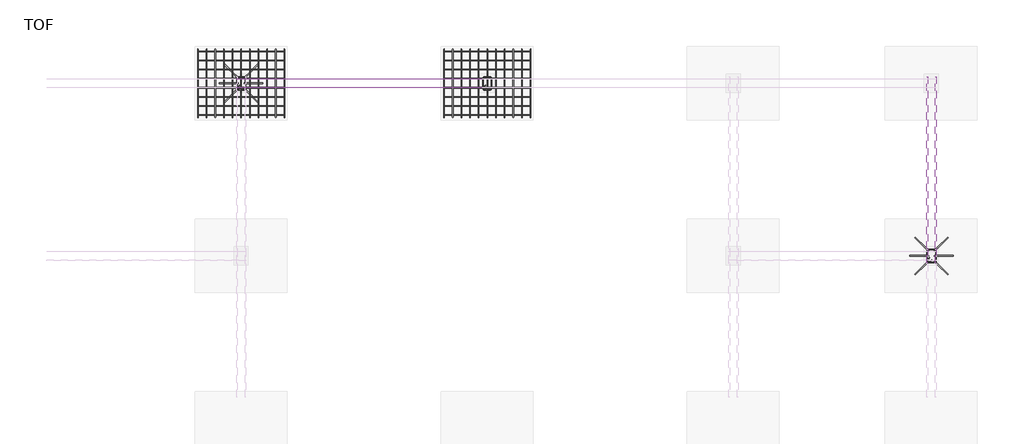
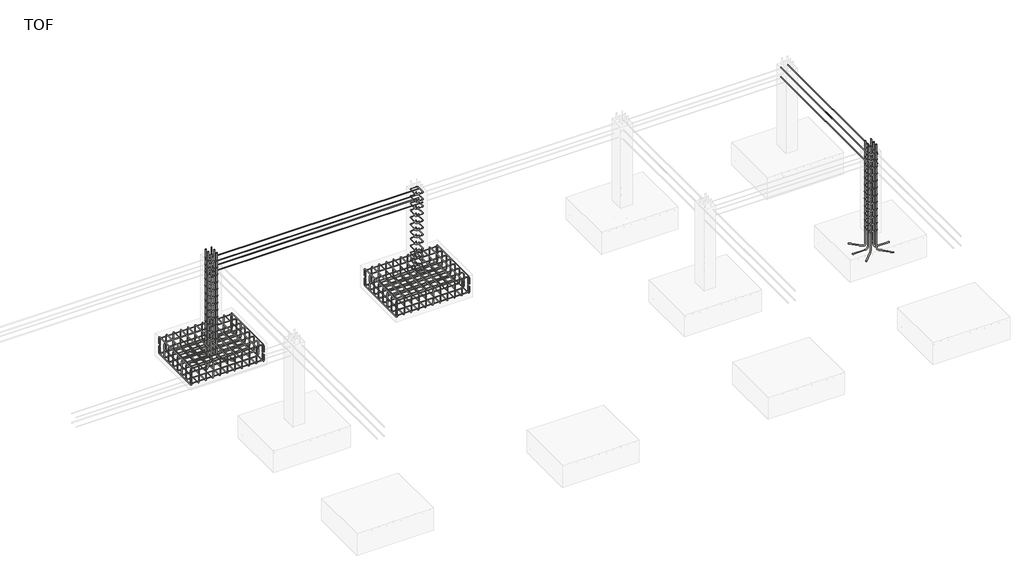
# One storey, part 9 of 10: 31 reinforcing bars.
"""IFC4 building model written with IfcOpenShell, lengths in millimetres."""

from ifc_helpers import new_model, si_unit, point, frame, origin, place, context, project, spatial, polyline, circle_curve, trimmed, segment, composite_curve, source, transform, mapped, element, save
from ifc_brep_helpers import swept_disk

model = new_model("IFC4")

# Units and contexts
model_context = context("Model", 3, world=origin())
ifc_project = project(units=[si_unit("LENGTHUNIT", "METRE", prefix="MILLI")], contexts=[model_context])

# Site, building, storey
site = spatial("IfcSite", under=ifc_project)
building = spatial("IfcBuilding", under=site)
storey = spatial("IfcBuildingStorey", under=building, Name="TOF", Elevation=-1828.8)

# Reinforcing bars
placement = place(None, origin())
reinforcing_bar_shape = source(origin(), model_context, "Body", "SolidModel", [
    swept_disk(composite_curve([segment(polyline([(2315.2782143, -7144.6267376, -2018.8), (2315.2782143, -7144.6267376, -1908.8)]), True, "CONTINUOUS"), segment(trimmed(circle_curve(frame((2315.2782143, -7179.6267376, -1908.8), z_axis=(1.0, 0.0, 0.0), x_axis=(0.0, 35.0, 0.0)), 35.0), [point((2315.2782143, -7144.6267376, -1908.8))], [point((2315.2782143, -7179.6267376, -1873.8))], True, "CARTESIAN"), True, "CONTINUOUS"), segment(polyline([(2315.2782143, -7179.6267376, -1873.8), (2315.2782143, -8219.6267376, -1873.8)]), True, "CONTINUOUS"), segment(trimmed(circle_curve(frame((2315.2782143, -8219.6267376, -1908.8), z_axis=(1.0, 0.0, 0.0), x_axis=(0.0, 0.0, 35.0)), 35.0), [point((2315.2782143, -8219.6267376, -1873.8))], [point((2315.2782143, -8254.6267376, -1908.8))], True, "CARTESIAN"), True, "CONTINUOUS"), segment(polyline([(2315.2782143, -8254.6267376, -1908.8), (2315.2782143, -8254.6267376, -2018.8)]), True, "CONTINUOUS")], self_intersect=False), 5.0),
])
element("IfcReinforcingBar", 1, at=placement, inside=storey, context=model_context, shape_type="MappedRepresentation", body=[
    mapped(reinforcing_bar_shape, transform((0.0, 0.0, 0.0), x_axis=(1.0, 0.0, 0.0), y_axis=(0.0, 1.0, 0.0), z_axis=(0.0, 0.0, 1.0))),
    mapped(reinforcing_bar_shape, transform((-141.0, 0.0, 0.0), x_axis=(1.0, 0.0, 0.0), y_axis=(0.0, 1.0, 0.0), z_axis=(0.0, 0.0, 1.0))),
    mapped(reinforcing_bar_shape, transform((-282.0, 0.0, 0.0), x_axis=(1.0, 0.0, 0.0), y_axis=(0.0, 1.0, 0.0), z_axis=(0.0, 0.0, 1.0))),
    mapped(reinforcing_bar_shape, transform((-423.0, 0.0, 0.0), x_axis=(1.0, 0.0, 0.0), y_axis=(0.0, 1.0, 0.0), z_axis=(0.0, 0.0, 1.0))),
    mapped(reinforcing_bar_shape, transform((-564.0, 0.0, 0.0), x_axis=(1.0, 0.0, 0.0), y_axis=(0.0, 1.0, 0.0), z_axis=(0.0, 0.0, 1.0))),
    mapped(reinforcing_bar_shape, transform((-705.0, 0.0, 0.0), x_axis=(1.0, 0.0, 0.0), y_axis=(0.0, 1.0, 0.0), z_axis=(0.0, 0.0, 1.0))),
    mapped(reinforcing_bar_shape, transform((-846.0, 0.0, 0.0), x_axis=(1.0, 0.0, 0.0), y_axis=(0.0, 1.0, 0.0), z_axis=(0.0, 0.0, 1.0))),
    mapped(reinforcing_bar_shape, transform((-987.0, 0.0, 0.0), x_axis=(1.0, 0.0, 0.0), y_axis=(0.0, 1.0, 0.0), z_axis=(0.0, 0.0, 1.0))),
    mapped(reinforcing_bar_shape, transform((-1128.0, 0.0, 0.0), x_axis=(1.0, 0.0, 0.0), y_axis=(0.0, 1.0, 0.0), z_axis=(0.0, 0.0, 1.0))),
    mapped(reinforcing_bar_shape, transform((-1269.0, 0.0, 0.0), x_axis=(1.0, 0.0, 0.0), y_axis=(0.0, 1.0, 0.0), z_axis=(0.0, 0.0, 1.0))),
    mapped(reinforcing_bar_shape, transform((-1410.0, 0.0, 0.0), x_axis=(1.0, 0.0, 0.0), y_axis=(0.0, 1.0, 0.0), z_axis=(0.0, 0.0, 1.0))),
])
reinforcing_bar_2_shape = source(origin(), model_context, "Body", "SolidModel", [
    swept_disk(composite_curve([segment(polyline([(2315.2782143, -8254.6267376, -2077.5233378), (2315.2782143, -8254.6267376, -2187.5233378)]), True, "CONTINUOUS"), segment(trimmed(circle_curve(frame((2315.2782143, -8219.6267376, -2187.5233378), z_axis=(1.0, 0.0, 0.0), x_axis=(0.0, -35.0, 0.0)), 35.0), [point((2315.2782143, -8254.6267376, -2187.5233378))], [point((2315.2782143, -8219.6267376, -2222.5233378))], True, "CARTESIAN"), True, "CONTINUOUS"), segment(polyline([(2315.2782143, -8219.6267376, -2222.5233378), (2315.2782143, -7179.6267376, -2222.5233378)]), True, "CONTINUOUS"), segment(trimmed(circle_curve(frame((2315.2782143, -7179.6267376, -2187.5233378), z_axis=(1.0, 0.0, 0.0), x_axis=(0.0, 0.0, -35.0)), 35.0), [point((2315.2782143, -7179.6267376, -2222.5233378))], [point((2315.2782143, -7144.6267376, -2187.5233378))], True, "CARTESIAN"), True, "CONTINUOUS"), segment(polyline([(2315.2782143, -7144.6267376, -2187.5233378), (2315.2782143, -7144.6267376, -2077.5233378)]), True, "CONTINUOUS")], self_intersect=False), 5.0),
])
element("IfcReinforcingBar", 2, at=placement, inside=storey, context=model_context, shape_type="MappedRepresentation", body=[
    mapped(reinforcing_bar_2_shape, transform((0.0, 0.0, 0.0), x_axis=(1.0, 0.0, 0.0), y_axis=(0.0, 1.0, 0.0), z_axis=(0.0, 0.0, 1.0))),
    mapped(reinforcing_bar_2_shape, transform((-141.0, 0.0, 0.0), x_axis=(1.0, 0.0, 0.0), y_axis=(0.0, 1.0, 0.0), z_axis=(0.0, 0.0, 1.0))),
    mapped(reinforcing_bar_2_shape, transform((-282.0, 0.0, 0.0), x_axis=(1.0, 0.0, 0.0), y_axis=(0.0, 1.0, 0.0), z_axis=(0.0, 0.0, 1.0))),
    mapped(reinforcing_bar_2_shape, transform((-423.0, 0.0, 0.0), x_axis=(1.0, 0.0, 0.0), y_axis=(0.0, 1.0, 0.0), z_axis=(0.0, 0.0, 1.0))),
    mapped(reinforcing_bar_2_shape, transform((-564.0, 0.0, 0.0), x_axis=(1.0, 0.0, 0.0), y_axis=(0.0, 1.0, 0.0), z_axis=(0.0, 0.0, 1.0))),
    mapped(reinforcing_bar_2_shape, transform((-705.0, 0.0, 0.0), x_axis=(1.0, 0.0, 0.0), y_axis=(0.0, 1.0, 0.0), z_axis=(0.0, 0.0, 1.0))),
    mapped(reinforcing_bar_2_shape, transform((-846.0, 0.0, 0.0), x_axis=(1.0, 0.0, 0.0), y_axis=(0.0, 1.0, 0.0), z_axis=(0.0, 0.0, 1.0))),
    mapped(reinforcing_bar_2_shape, transform((-987.0, 0.0, 0.0), x_axis=(1.0, 0.0, 0.0), y_axis=(0.0, 1.0, 0.0), z_axis=(0.0, 0.0, 1.0))),
    mapped(reinforcing_bar_2_shape, transform((-1128.0, 0.0, 0.0), x_axis=(1.0, 0.0, 0.0), y_axis=(0.0, 1.0, 0.0), z_axis=(0.0, 0.0, 1.0))),
    mapped(reinforcing_bar_2_shape, transform((-1269.0, 0.0, 0.0), x_axis=(1.0, 0.0, 0.0), y_axis=(0.0, 1.0, 0.0), z_axis=(0.0, 0.0, 1.0))),
    mapped(reinforcing_bar_2_shape, transform((-1410.0, 0.0, 0.0), x_axis=(1.0, 0.0, 0.0), y_axis=(0.0, 1.0, 0.0), z_axis=(0.0, 0.0, 1.0))),
])
reinforcing_bar_3_shape = source(origin(), model_context, "Body", "SolidModel", [
    swept_disk(composite_curve([segment(polyline([(2315.2782143, -7179.6861459, -2066.1776706), (2315.2782143, -7179.6861459, -2176.1776706)]), True, "CONTINUOUS"), segment(trimmed(circle_curve(frame((2280.2782143, -7179.6861459, -2176.1776706), z_axis=(0.0, 1.0, 0.0), x_axis=(35.0, 0.0, 0.0)), 35.0), [point((2315.2782143, -7179.6861459, -2176.1776706))], [point((2280.2782143, -7179.6861459, -2211.1776706))], True, "CARTESIAN"), True, "CONTINUOUS"), segment(polyline([(2280.2782143, -7179.6861459, -2211.1776706), (940.2782143, -7179.6861459, -2211.1776706)]), True, "CONTINUOUS"), segment(trimmed(circle_curve(frame((940.2782143, -7179.6861459, -2176.1776706), z_axis=(0.0, 1.0, 0.0), x_axis=(0.0, 0.0, -35.0)), 35.0), [point((940.2782143, -7179.6861459, -2211.1776706))], [point((905.2782143, -7179.6861459, -2176.1776706))], True, "CARTESIAN"), True, "CONTINUOUS"), segment(polyline([(905.2782143, -7179.6861459, -2176.1776706), (905.2782143, -7179.6861459, -2066.1776706)]), True, "CONTINUOUS")], self_intersect=False), 5.0),
])
element("IfcReinforcingBar", 3, at=placement, inside=storey, context=model_context, shape_type="MappedRepresentation", body=[
    mapped(reinforcing_bar_3_shape, transform((0.0, 0.0, 0.0), x_axis=(1.0, 0.0, 0.0), y_axis=(0.0, 1.0, 0.0), z_axis=(0.0, 0.0, 1.0))),
    mapped(reinforcing_bar_3_shape, transform((0.0, -148.0321606, 0.0), x_axis=(1.0, 0.0, 0.0), y_axis=(0.0, 1.0, 0.0), z_axis=(0.0, 0.0, 1.0))),
    mapped(reinforcing_bar_3_shape, transform((0.0, -296.0643211, 0.0), x_axis=(1.0, 0.0, 0.0), y_axis=(0.0, 1.0, 0.0), z_axis=(0.0, 0.0, 1.0))),
    mapped(reinforcing_bar_3_shape, transform((0.0, -444.0964817, 0.0), x_axis=(1.0, 0.0, 0.0), y_axis=(0.0, 1.0, 0.0), z_axis=(0.0, 0.0, 1.0))),
    mapped(reinforcing_bar_3_shape, transform((0.0, -592.1286423, 0.0), x_axis=(1.0, 0.0, 0.0), y_axis=(0.0, 1.0, 0.0), z_axis=(0.0, 0.0, 1.0))),
    mapped(reinforcing_bar_3_shape, transform((0.0, -740.1608029, 0.0), x_axis=(1.0, 0.0, 0.0), y_axis=(0.0, 1.0, 0.0), z_axis=(0.0, 0.0, 1.0))),
    mapped(reinforcing_bar_3_shape, transform((0.0, -888.1929634, 0.0), x_axis=(1.0, 0.0, 0.0), y_axis=(0.0, 1.0, 0.0), z_axis=(0.0, 0.0, 1.0))),
    mapped(reinforcing_bar_3_shape, transform((0.0, -1036.225124, 0.0), x_axis=(1.0, 0.0, 0.0), y_axis=(0.0, 1.0, 0.0), z_axis=(0.0, 0.0, 1.0))),
])
reinforcing_bar_4_shape = source(origin(), model_context, "Body", "SolidModel", [
    swept_disk(composite_curve([segment(polyline([(2315.2782143, -8215.9112699, -2039.256778), (2315.2782143, -8215.9112699, -1929.256778)]), True, "CONTINUOUS"), segment(trimmed(circle_curve(frame((2280.2782143, -8215.9112699, -1929.256778), z_axis=(0.0, -1.0, 0.0), x_axis=(35.0, 0.0, 0.0)), 35.0), [point((2315.2782143, -8215.9112699, -1929.256778))], [point((2280.2782143, -8215.9112699, -1894.256778))], True, "CARTESIAN"), True, "CONTINUOUS"), segment(polyline([(2280.2782143, -8215.9112699, -1894.256778), (940.2782143, -8215.9112699, -1894.256778)]), True, "CONTINUOUS"), segment(trimmed(circle_curve(frame((940.2782143, -8215.9112699, -1929.256778), z_axis=(0.0, -1.0, 0.0), x_axis=(0.0, 0.0, 35.0)), 35.0), [point((940.2782143, -8215.9112699, -1894.256778))], [point((905.2782143, -8215.9112699, -1929.256778))], True, "CARTESIAN"), True, "CONTINUOUS"), segment(polyline([(905.2782143, -8215.9112699, -1929.256778), (905.2782143, -8215.9112699, -2039.256778)]), True, "CONTINUOUS")], self_intersect=False), 5.0),
])
element("IfcReinforcingBar", 4, at=placement, inside=storey, context=model_context, shape_type="MappedRepresentation", body=[
    mapped(reinforcing_bar_4_shape, transform((0.0, 0.0, 0.0), x_axis=(1.0, 0.0, 0.0), y_axis=(0.0, 1.0, 0.0), z_axis=(0.0, 0.0, 1.0))),
    mapped(reinforcing_bar_4_shape, transform((0.0, 148.0321606, 0.0), x_axis=(1.0, 0.0, 0.0), y_axis=(0.0, 1.0, 0.0), z_axis=(0.0, 0.0, 1.0))),
    mapped(reinforcing_bar_4_shape, transform((0.0, 296.0643211, 0.0), x_axis=(1.0, 0.0, 0.0), y_axis=(0.0, 1.0, 0.0), z_axis=(0.0, 0.0, 1.0))),
    mapped(reinforcing_bar_4_shape, transform((0.0, 444.0964817, 0.0), x_axis=(1.0, 0.0, 0.0), y_axis=(0.0, 1.0, 0.0), z_axis=(0.0, 0.0, 1.0))),
    mapped(reinforcing_bar_4_shape, transform((0.0, 592.1286423, 0.0), x_axis=(1.0, 0.0, 0.0), y_axis=(0.0, 1.0, 0.0), z_axis=(0.0, 0.0, 1.0))),
    mapped(reinforcing_bar_4_shape, transform((0.0, 740.1608029, 0.0), x_axis=(1.0, 0.0, 0.0), y_axis=(0.0, 1.0, 0.0), z_axis=(0.0, 0.0, 1.0))),
    mapped(reinforcing_bar_4_shape, transform((0.0, 888.1929634, 0.0), x_axis=(1.0, 0.0, 0.0), y_axis=(0.0, 1.0, 0.0), z_axis=(0.0, 0.0, 1.0))),
    mapped(reinforcing_bar_4_shape, transform((0.0, 1036.225124, 0.0), x_axis=(1.0, 0.0, 0.0), y_axis=(0.0, 1.0, 0.0), z_axis=(0.0, 0.0, 1.0))),
])
reinforcing_bar_5_shape = source(origin(), model_context, "Body", "SolidModel", [
    swept_disk(composite_curve([segment(polyline([(6330.2782143, -7144.6267376, -2018.8), (6330.2782143, -7144.6267376, -1908.8)]), True, "CONTINUOUS"), segment(trimmed(circle_curve(frame((6330.2782143, -7179.6267376, -1908.8), z_axis=(1.0, 0.0, 0.0), x_axis=(0.0, 35.0, 0.0)), 35.0), [point((6330.2782143, -7144.6267376, -1908.8))], [point((6330.2782143, -7179.6267376, -1873.8))], True, "CARTESIAN"), True, "CONTINUOUS"), segment(polyline([(6330.2782143, -7179.6267376, -1873.8), (6330.2782143, -8219.6267376, -1873.8)]), True, "CONTINUOUS"), segment(trimmed(circle_curve(frame((6330.2782143, -8219.6267376, -1908.8), z_axis=(1.0, 0.0, 0.0), x_axis=(0.0, 0.0, 35.0)), 35.0), [point((6330.2782143, -8219.6267376, -1873.8))], [point((6330.2782143, -8254.6267376, -1908.8))], True, "CARTESIAN"), True, "CONTINUOUS"), segment(polyline([(6330.2782143, -8254.6267376, -1908.8), (6330.2782143, -8254.6267376, -2018.8)]), True, "CONTINUOUS")], self_intersect=False), 5.0),
])
element("IfcReinforcingBar", 5, at=placement, inside=storey, context=model_context, shape_type="MappedRepresentation", body=[
    mapped(reinforcing_bar_5_shape, transform((0.0, 0.0, 0.0), x_axis=(1.0, 0.0, 0.0), y_axis=(0.0, 1.0, 0.0), z_axis=(0.0, 0.0, 1.0))),
    mapped(reinforcing_bar_5_shape, transform((-141.0, 0.0, 0.0), x_axis=(1.0, 0.0, 0.0), y_axis=(0.0, 1.0, 0.0), z_axis=(0.0, 0.0, 1.0))),
    mapped(reinforcing_bar_5_shape, transform((-282.0, 0.0, 0.0), x_axis=(1.0, 0.0, 0.0), y_axis=(0.0, 1.0, 0.0), z_axis=(0.0, 0.0, 1.0))),
    mapped(reinforcing_bar_5_shape, transform((-423.0, 0.0, 0.0), x_axis=(1.0, 0.0, 0.0), y_axis=(0.0, 1.0, 0.0), z_axis=(0.0, 0.0, 1.0))),
    mapped(reinforcing_bar_5_shape, transform((-564.0, 0.0, 0.0), x_axis=(1.0, 0.0, 0.0), y_axis=(0.0, 1.0, 0.0), z_axis=(0.0, 0.0, 1.0))),
    mapped(reinforcing_bar_5_shape, transform((-705.0, 0.0, 0.0), x_axis=(1.0, 0.0, 0.0), y_axis=(0.0, 1.0, 0.0), z_axis=(0.0, 0.0, 1.0))),
    mapped(reinforcing_bar_5_shape, transform((-846.0, 0.0, 0.0), x_axis=(1.0, 0.0, 0.0), y_axis=(0.0, 1.0, 0.0), z_axis=(0.0, 0.0, 1.0))),
    mapped(reinforcing_bar_5_shape, transform((-987.0, 0.0, 0.0), x_axis=(1.0, 0.0, 0.0), y_axis=(0.0, 1.0, 0.0), z_axis=(0.0, 0.0, 1.0))),
    mapped(reinforcing_bar_5_shape, transform((-1128.0, 0.0, 0.0), x_axis=(1.0, 0.0, 0.0), y_axis=(0.0, 1.0, 0.0), z_axis=(0.0, 0.0, 1.0))),
    mapped(reinforcing_bar_5_shape, transform((-1269.0, 0.0, 0.0), x_axis=(1.0, 0.0, 0.0), y_axis=(0.0, 1.0, 0.0), z_axis=(0.0, 0.0, 1.0))),
    mapped(reinforcing_bar_5_shape, transform((-1410.0, 0.0, 0.0), x_axis=(1.0, 0.0, 0.0), y_axis=(0.0, 1.0, 0.0), z_axis=(0.0, 0.0, 1.0))),
])
reinforcing_bar_6_shape = source(origin(), model_context, "Body", "SolidModel", [
    swept_disk(composite_curve([segment(polyline([(6330.2782143, -8254.6267376, -2077.5233378), (6330.2782143, -8254.6267376, -2187.5233378)]), True, "CONTINUOUS"), segment(trimmed(circle_curve(frame((6330.2782143, -8219.6267376, -2187.5233378), z_axis=(1.0, 0.0, 0.0), x_axis=(0.0, -35.0, 0.0)), 35.0), [point((6330.2782143, -8254.6267376, -2187.5233378))], [point((6330.2782143, -8219.6267376, -2222.5233378))], True, "CARTESIAN"), True, "CONTINUOUS"), segment(polyline([(6330.2782143, -8219.6267376, -2222.5233378), (6330.2782143, -7179.6267376, -2222.5233378)]), True, "CONTINUOUS"), segment(trimmed(circle_curve(frame((6330.2782143, -7179.6267376, -2187.5233378), z_axis=(1.0, 0.0, 0.0), x_axis=(0.0, 0.0, -35.0)), 35.0), [point((6330.2782143, -7179.6267376, -2222.5233378))], [point((6330.2782143, -7144.6267376, -2187.5233378))], True, "CARTESIAN"), True, "CONTINUOUS"), segment(polyline([(6330.2782143, -7144.6267376, -2187.5233378), (6330.2782143, -7144.6267376, -2077.5233378)]), True, "CONTINUOUS")], self_intersect=False), 5.0),
])
element("IfcReinforcingBar", 6, at=placement, inside=storey, context=model_context, shape_type="MappedRepresentation", body=[
    mapped(reinforcing_bar_6_shape, transform((0.0, 0.0, 0.0), x_axis=(1.0, 0.0, 0.0), y_axis=(0.0, 1.0, 0.0), z_axis=(0.0, 0.0, 1.0))),
    mapped(reinforcing_bar_6_shape, transform((-141.0, 0.0, 0.0), x_axis=(1.0, 0.0, 0.0), y_axis=(0.0, 1.0, 0.0), z_axis=(0.0, 0.0, 1.0))),
    mapped(reinforcing_bar_6_shape, transform((-282.0, 0.0, 0.0), x_axis=(1.0, 0.0, 0.0), y_axis=(0.0, 1.0, 0.0), z_axis=(0.0, 0.0, 1.0))),
    mapped(reinforcing_bar_6_shape, transform((-423.0, 0.0, 0.0), x_axis=(1.0, 0.0, 0.0), y_axis=(0.0, 1.0, 0.0), z_axis=(0.0, 0.0, 1.0))),
    mapped(reinforcing_bar_6_shape, transform((-564.0, 0.0, 0.0), x_axis=(1.0, 0.0, 0.0), y_axis=(0.0, 1.0, 0.0), z_axis=(0.0, 0.0, 1.0))),
    mapped(reinforcing_bar_6_shape, transform((-705.0, 0.0, 0.0), x_axis=(1.0, 0.0, 0.0), y_axis=(0.0, 1.0, 0.0), z_axis=(0.0, 0.0, 1.0))),
    mapped(reinforcing_bar_6_shape, transform((-846.0, 0.0, 0.0), x_axis=(1.0, 0.0, 0.0), y_axis=(0.0, 1.0, 0.0), z_axis=(0.0, 0.0, 1.0))),
    mapped(reinforcing_bar_6_shape, transform((-987.0, 0.0, 0.0), x_axis=(1.0, 0.0, 0.0), y_axis=(0.0, 1.0, 0.0), z_axis=(0.0, 0.0, 1.0))),
    mapped(reinforcing_bar_6_shape, transform((-1128.0, 0.0, 0.0), x_axis=(1.0, 0.0, 0.0), y_axis=(0.0, 1.0, 0.0), z_axis=(0.0, 0.0, 1.0))),
    mapped(reinforcing_bar_6_shape, transform((-1269.0, 0.0, 0.0), x_axis=(1.0, 0.0, 0.0), y_axis=(0.0, 1.0, 0.0), z_axis=(0.0, 0.0, 1.0))),
    mapped(reinforcing_bar_6_shape, transform((-1410.0, 0.0, 0.0), x_axis=(1.0, 0.0, 0.0), y_axis=(0.0, 1.0, 0.0), z_axis=(0.0, 0.0, 1.0))),
])
reinforcing_bar_7_shape = source(origin(), model_context, "Body", "SolidModel", [
    swept_disk(composite_curve([segment(polyline([(6330.2782143, -7179.6861459, -2066.1776706), (6330.2782143, -7179.6861459, -2176.1776706)]), True, "CONTINUOUS"), segment(trimmed(circle_curve(frame((6295.2782143, -7179.6861459, -2176.1776706), z_axis=(0.0, 1.0, 0.0), x_axis=(35.0, 0.0, 0.0)), 35.0), [point((6330.2782143, -7179.6861459, -2176.1776706))], [point((6295.2782143, -7179.6861459, -2211.1776706))], True, "CARTESIAN"), True, "CONTINUOUS"), segment(polyline([(6295.2782143, -7179.6861459, -2211.1776706), (4955.2782143, -7179.6861459, -2211.1776706)]), True, "CONTINUOUS"), segment(trimmed(circle_curve(frame((4955.2782143, -7179.6861459, -2176.1776706), z_axis=(0.0, 1.0, 0.0), x_axis=(0.0, 0.0, -35.0)), 35.0), [point((4955.2782143, -7179.6861459, -2211.1776706))], [point((4920.2782143, -7179.6861459, -2176.1776706))], True, "CARTESIAN"), True, "CONTINUOUS"), segment(polyline([(4920.2782143, -7179.6861459, -2176.1776706), (4920.2782143, -7179.6861459, -2066.1776706)]), True, "CONTINUOUS")], self_intersect=False), 5.0),
])
element("IfcReinforcingBar", 7, at=placement, inside=storey, context=model_context, shape_type="MappedRepresentation", body=[
    mapped(reinforcing_bar_7_shape, transform((0.0, 0.0, 0.0), x_axis=(1.0, 0.0, 0.0), y_axis=(0.0, 1.0, 0.0), z_axis=(0.0, 0.0, 1.0))),
    mapped(reinforcing_bar_7_shape, transform((0.0, -148.0321606, 0.0), x_axis=(1.0, 0.0, 0.0), y_axis=(0.0, 1.0, 0.0), z_axis=(0.0, 0.0, 1.0))),
    mapped(reinforcing_bar_7_shape, transform((0.0, -296.0643211, 0.0), x_axis=(1.0, 0.0, 0.0), y_axis=(0.0, 1.0, 0.0), z_axis=(0.0, 0.0, 1.0))),
    mapped(reinforcing_bar_7_shape, transform((0.0, -444.0964817, 0.0), x_axis=(1.0, 0.0, 0.0), y_axis=(0.0, 1.0, 0.0), z_axis=(0.0, 0.0, 1.0))),
    mapped(reinforcing_bar_7_shape, transform((0.0, -592.1286423, 0.0), x_axis=(1.0, 0.0, 0.0), y_axis=(0.0, 1.0, 0.0), z_axis=(0.0, 0.0, 1.0))),
    mapped(reinforcing_bar_7_shape, transform((0.0, -740.1608029, 0.0), x_axis=(1.0, 0.0, 0.0), y_axis=(0.0, 1.0, 0.0), z_axis=(0.0, 0.0, 1.0))),
    mapped(reinforcing_bar_7_shape, transform((0.0, -888.1929634, 0.0), x_axis=(1.0, 0.0, 0.0), y_axis=(0.0, 1.0, 0.0), z_axis=(0.0, 0.0, 1.0))),
    mapped(reinforcing_bar_7_shape, transform((0.0, -1036.225124, 0.0), x_axis=(1.0, 0.0, 0.0), y_axis=(0.0, 1.0, 0.0), z_axis=(0.0, 0.0, 1.0))),
])
reinforcing_bar_8_shape = source(origin(), model_context, "Body", "SolidModel", [
    swept_disk(composite_curve([segment(polyline([(6330.2782143, -8215.9112699, -2039.256778), (6330.2782143, -8215.9112699, -1929.256778)]), True, "CONTINUOUS"), segment(trimmed(circle_curve(frame((6295.2782143, -8215.9112699, -1929.256778), z_axis=(0.0, -1.0, 0.0), x_axis=(35.0, 0.0, 0.0)), 35.0), [point((6330.2782143, -8215.9112699, -1929.256778))], [point((6295.2782143, -8215.9112699, -1894.256778))], True, "CARTESIAN"), True, "CONTINUOUS"), segment(polyline([(6295.2782143, -8215.9112699, -1894.256778), (4955.2782143, -8215.9112699, -1894.256778)]), True, "CONTINUOUS"), segment(trimmed(circle_curve(frame((4955.2782143, -8215.9112699, -1929.256778), z_axis=(0.0, -1.0, 0.0), x_axis=(0.0, 0.0, 35.0)), 35.0), [point((4955.2782143, -8215.9112699, -1894.256778))], [point((4920.2782143, -8215.9112699, -1929.256778))], True, "CARTESIAN"), True, "CONTINUOUS"), segment(polyline([(4920.2782143, -8215.9112699, -1929.256778), (4920.2782143, -8215.9112699, -2039.256778)]), True, "CONTINUOUS")], self_intersect=False), 5.0),
])
element("IfcReinforcingBar", 8, at=placement, inside=storey, context=model_context, shape_type="MappedRepresentation", body=[
    mapped(reinforcing_bar_8_shape, transform((0.0, 0.0, 0.0), x_axis=(1.0, 0.0, 0.0), y_axis=(0.0, 1.0, 0.0), z_axis=(0.0, 0.0, 1.0))),
    mapped(reinforcing_bar_8_shape, transform((0.0, 148.0321606, 0.0), x_axis=(1.0, 0.0, 0.0), y_axis=(0.0, 1.0, 0.0), z_axis=(0.0, 0.0, 1.0))),
    mapped(reinforcing_bar_8_shape, transform((0.0, 296.0643211, 0.0), x_axis=(1.0, 0.0, 0.0), y_axis=(0.0, 1.0, 0.0), z_axis=(0.0, 0.0, 1.0))),
    mapped(reinforcing_bar_8_shape, transform((0.0, 444.0964817, 0.0), x_axis=(1.0, 0.0, 0.0), y_axis=(0.0, 1.0, 0.0), z_axis=(0.0, 0.0, 1.0))),
    mapped(reinforcing_bar_8_shape, transform((0.0, 592.1286423, 0.0), x_axis=(1.0, 0.0, 0.0), y_axis=(0.0, 1.0, 0.0), z_axis=(0.0, 0.0, 1.0))),
    mapped(reinforcing_bar_8_shape, transform((0.0, 740.1608029, 0.0), x_axis=(1.0, 0.0, 0.0), y_axis=(0.0, 1.0, 0.0), z_axis=(0.0, 0.0, 1.0))),
    mapped(reinforcing_bar_8_shape, transform((0.0, 888.1929634, 0.0), x_axis=(1.0, 0.0, 0.0), y_axis=(0.0, 1.0, 0.0), z_axis=(0.0, 0.0, 1.0))),
    mapped(reinforcing_bar_8_shape, transform((0.0, 1036.225124, 0.0), x_axis=(1.0, 0.0, 0.0), y_axis=(0.0, 1.0, 0.0), z_axis=(0.0, 0.0, 1.0))),
])
reinforcing_bar_9_shape = source(origin(), model_context, "Body", "SolidModel", [
    swept_disk(composite_curve([segment(polyline([(12840.248777, -10545.7150493, -1784.8), (12806.3076515, -10579.6561748, -1784.8)]), True, "CONTINUOUS"), segment(trimmed(circle_curve(frame((12823.2782143, -10596.6267376, -1784.8), z_axis=(0.0, 0.0, 1.0), x_axis=(-16.970562800001062, 16.970562799999243, 0.0)), 24.0), [point((12806.3076515, -10579.6561748, -1784.8))], [point((12823.2782143, -10620.6267376, -1784.8))], True, "CARTESIAN"), True, "CONTINUOUS"), segment(polyline([(12823.2782143, -10620.6267376, -1784.8), (12917.2782143, -10620.6267376, -1784.8)]), True, "CONTINUOUS"), segment(trimmed(circle_curve(frame((12917.2782143, -10596.6267376, -1784.8), z_axis=(0.0, 0.0, 1.0), x_axis=(0.0, -24.0, 0.0)), 24.0), [point((12917.2782143, -10620.6267376, -1784.8))], [point((12941.2782143, -10596.6267376, -1784.8))], True, "CARTESIAN"), True, "CONTINUOUS"), segment(polyline([(12941.2782143, -10596.6267376, -1784.8), (12941.2782143, -10432.6267376, -1784.8)]), True, "CONTINUOUS"), segment(trimmed(circle_curve(frame((12917.3162115, -10432.6267376, -1786.149972), z_axis=(-0.05624883273897078, 0.0, 0.9984167811167355), x_axis=(23.962002800000846, 0.0, 1.3499719999999797)), 24.0), [point((12941.2782143, -10432.6267376, -1784.8))], [point((12917.3162115, -10408.6267376, -1786.149972))], True, "CARTESIAN"), True, "CONTINUOUS"), segment(polyline([(12917.3162115, -10408.6267376, -1786.149972), (12823.240217, -10408.6267376, -1791.450028)]), True, "CONTINUOUS"), segment(trimmed(circle_curve(frame((12823.240217, -10432.6267376, -1791.450028), z_axis=(-0.05624883273897078, 0.0, 0.9984167811167355), x_axis=(0.0, 24.0, 0.0)), 24.0), [point((12823.240217, -10408.6267376, -1791.450028))], [point((12799.2782143, -10432.6267376, -1792.8))], True, "CARTESIAN"), True, "CONTINUOUS"), segment(polyline([(12799.2782143, -10432.6267376, -1792.8), (12799.2782143, -10596.6267376, -1792.8)]), True, "CONTINUOUS"), segment(trimmed(circle_curve(frame((12823.2782143, -10596.6267376, -1792.8), z_axis=(0.0, 0.0, 1.0), x_axis=(-24.0, 0.0, 0.0)), 24.0), [point((12799.2782143, -10596.6267376, -1792.8))], [point((12840.248777, -10613.5973003, -1792.8))], True, "CARTESIAN"), True, "CONTINUOUS"), segment(polyline([(12840.248777, -10613.5973003, -1792.8), (12874.1899025, -10579.6561748, -1792.8)]), True, "CONTINUOUS")], self_intersect=False), 4.0),
])
element("IfcReinforcingBar", 9, at=placement, inside=storey, context=model_context, shape_type="MappedRepresentation", body=[
    mapped(reinforcing_bar_9_shape, transform((0.0, 0.0, 0.0), x_axis=(1.0, 0.0, 0.0), y_axis=(0.0, 1.0, 0.0), z_axis=(0.0, 0.0, 1.0))),
    mapped(reinforcing_bar_9_shape, transform((0.0, 0.0, 145.9395608), x_axis=(1.0, 0.0, 0.0), y_axis=(0.0, 1.0, 0.0), z_axis=(0.0, 0.0, 1.0))),
    mapped(reinforcing_bar_9_shape, transform((0.0, 0.0, 291.8791216), x_axis=(1.0, 0.0, 0.0), y_axis=(0.0, 1.0, 0.0), z_axis=(0.0, 0.0, 1.0))),
    mapped(reinforcing_bar_9_shape, transform((0.0, 0.0, 437.8186825), x_axis=(1.0, 0.0, 0.0), y_axis=(0.0, 1.0, 0.0), z_axis=(0.0, 0.0, 1.0))),
    mapped(reinforcing_bar_9_shape, transform((0.0, 0.0, 583.7582433), x_axis=(1.0, 0.0, 0.0), y_axis=(0.0, 1.0, 0.0), z_axis=(0.0, 0.0, 1.0))),
    mapped(reinforcing_bar_9_shape, transform((0.0, 0.0, 729.6978041), x_axis=(1.0, 0.0, 0.0), y_axis=(0.0, 1.0, 0.0), z_axis=(0.0, 0.0, 1.0))),
    mapped(reinforcing_bar_9_shape, transform((0.0, 0.0, 875.6373649), x_axis=(1.0, 0.0, 0.0), y_axis=(0.0, 1.0, 0.0), z_axis=(0.0, 0.0, 1.0))),
    mapped(reinforcing_bar_9_shape, transform((0.0, 0.0, 1021.5769258), x_axis=(1.0, 0.0, 0.0), y_axis=(0.0, 1.0, 0.0), z_axis=(0.0, 0.0, 1.0))),
    mapped(reinforcing_bar_9_shape, transform((0.0, 0.0, 1167.5164866), x_axis=(1.0, 0.0, 0.0), y_axis=(0.0, 1.0, 0.0), z_axis=(0.0, 0.0, 1.0))),
    mapped(reinforcing_bar_9_shape, transform((0.0, 0.0, 1313.4560474), x_axis=(1.0, 0.0, 0.0), y_axis=(0.0, 1.0, 0.0), z_axis=(0.0, 0.0, 1.0))),
    mapped(reinforcing_bar_9_shape, transform((0.0, 0.0, 1459.3956082), x_axis=(1.0, 0.0, 0.0), y_axis=(0.0, 1.0, 0.0), z_axis=(0.0, 0.0, 1.0))),
    mapped(reinforcing_bar_9_shape, transform((0.0, 0.0, 1605.3351691), x_axis=(1.0, 0.0, 0.0), y_axis=(0.0, 1.0, 0.0), z_axis=(0.0, 0.0, 1.0))),
])
element("IfcReinforcingBar", 10, at=placement, inside=storey, context=model_context, shape_type="SolidModel", body=[
    swept_disk(composite_curve([segment(polyline([(12925.884816, -10605.2333393, -20.0), (12925.884816, -10605.2333393, -2138.7824747)]), True, "CONTINUOUS"), segment(trimmed(circle_curve(frame((12965.1292424, -10644.4777657, -2138.7824747), z_axis=(-0.7071067811865545, -0.7071067811865406, 0.0), x_axis=(-39.24442640000052, 39.2444263999987, 0.0)), 55.5), [point((12925.884816, -10605.2333393, -2138.7824747))], [point((12965.1292424, -10644.4777657, -2194.2824747))], True, "CARTESIAN"), True, "CONTINUOUS"), segment(polyline([(12965.1292424, -10644.4777657, -2194.2824747), (13137.5083915, -10816.8569148, -2194.2824747)]), True, "CONTINUOUS")], self_intersect=False), 8.0),
])
element("IfcReinforcingBar", 11, at=placement, inside=storey, context=model_context, shape_type="SolidModel", body=[
    swept_disk(composite_curve([segment(polyline([(12925.934816, -10514.6267376, -20.0), (12925.934816, -10514.6267376, -2138.7824747)]), True, "CONTINUOUS"), segment(trimmed(circle_curve(frame((12981.434816, -10514.6267376, -2138.7824747), z_axis=(0.0, -1.0, 0.0), x_axis=(-55.5, 0.0, 0.0)), 55.5), [point((12925.934816, -10514.6267376, -2138.7824747))], [point((12981.434816, -10514.6267376, -2194.2824747))], True, "CARTESIAN"), True, "CONTINUOUS"), segment(polyline([(12981.434816, -10514.6267376, -2194.2824747), (13225.1657466, -10514.6267376, -2194.2824747)]), True, "CONTINUOUS")], self_intersect=False), 8.0),
])
element("IfcReinforcingBar", 12, at=placement, inside=storey, context=model_context, shape_type="SolidModel", body=[
    swept_disk(composite_curve([segment(polyline([(12925.884816, -10424.0201359, -20.0), (12925.884816, -10424.0201359, -2138.7824747)]), True, "CONTINUOUS"), segment(trimmed(circle_curve(frame((12965.1292424, -10384.7757095, -2138.7824747), z_axis=(0.7071067811865545, -0.7071067811865407, 0.0), x_axis=(-39.24442640000052, -39.24442640000052, 0.0)), 55.5), [point((12925.884816, -10424.0201359, -2138.7824747))], [point((12965.1292424, -10384.7757095, -2194.2824747))], True, "CARTESIAN"), True, "CONTINUOUS"), segment(polyline([(12965.1292424, -10384.7757095, -2194.2824747), (13137.5083915, -10212.3965603, -2194.2824747)]), True, "CONTINUOUS")], self_intersect=False), 8.0),
])
element("IfcReinforcingBar", 13, at=placement, inside=storey, context=model_context, shape_type="SolidModel", body=[
    swept_disk(composite_curve([segment(polyline([(12814.6716126, -10605.2333393, -20.0), (12814.6716126, -10605.2333393, -2138.7824747)]), True, "CONTINUOUS"), segment(trimmed(circle_curve(frame((12775.4271862, -10644.4777657, -2138.7824747), z_axis=(-0.7071067811865517, 0.7071067811865434, 0.0), x_axis=(39.2444263999987, 39.2444263999987, 0.0)), 55.5), [point((12814.6716126, -10605.2333393, -2138.7824747))], [point((12775.4271862, -10644.4777657, -2194.2824747))], True, "CARTESIAN"), True, "CONTINUOUS"), segment(polyline([(12775.4271862, -10644.4777657, -2194.2824747), (12603.048037, -10816.8569148, -2194.2824747)]), True, "CONTINUOUS")], self_intersect=False), 8.0),
])
element("IfcReinforcingBar", 14, at=placement, inside=storey, context=model_context, shape_type="SolidModel", body=[
    swept_disk(composite_curve([segment(polyline([(12814.6216126, -10514.6267376, -20.0), (12814.6216126, -10514.6267376, -2138.7824747)]), True, "CONTINUOUS"), segment(trimmed(circle_curve(frame((12759.1216126, -10514.6267376, -2138.7824747), z_axis=(0.0, 1.0, 0.0), x_axis=(55.5, 0.0, 0.0)), 55.5), [point((12814.6216126, -10514.6267376, -2138.7824747))], [point((12759.1216126, -10514.6267376, -2194.2824747))], True, "CARTESIAN"), True, "CONTINUOUS"), segment(polyline([(12759.1216126, -10514.6267376, -2194.2824747), (12515.3906819, -10514.6267376, -2194.2824747)]), True, "CONTINUOUS")], self_intersect=False), 8.0),
])
element("IfcReinforcingBar", 15, at=placement, inside=storey, context=model_context, shape_type="SolidModel", body=[
    swept_disk(composite_curve([segment(polyline([(12814.6716126, -10424.0201359, -20.0), (12814.6716126, -10424.0201359, -2138.7824747)]), True, "CONTINUOUS"), segment(trimmed(circle_curve(frame((12775.4271862, -10384.7757095, -2138.7824747), z_axis=(0.7071067811865572, 0.7071067811865379, 0.0), x_axis=(39.2444263999987, -39.24442640000052, 0.0)), 55.5), [point((12814.6716126, -10424.0201359, -2138.7824747))], [point((12775.4271862, -10384.7757095, -2194.2824747))], True, "CARTESIAN"), True, "CONTINUOUS"), segment(polyline([(12775.4271862, -10384.7757095, -2194.2824747), (12603.048037, -10212.3965603, -2194.2824747)]), True, "CONTINUOUS")], self_intersect=False), 8.0),
])
reinforcing_bar_10_shape = source(origin(), model_context, "Body", "SolidModel", [
    swept_disk(composite_curve([segment(polyline([(1580.248777, -7730.7150493, -1784.8), (1546.3076515, -7764.6561748, -1784.8)]), True, "CONTINUOUS"), segment(trimmed(circle_curve(frame((1563.2782143, -7781.6267376, -1784.8), z_axis=(0.0, 0.0, 1.0), x_axis=(-16.970562799999925, 16.970562799999243, 0.0)), 24.0), [point((1546.3076515, -7764.6561748, -1784.8))], [point((1563.2782143, -7805.6267376, -1784.8))], True, "CARTESIAN"), True, "CONTINUOUS"), segment(polyline([(1563.2782143, -7805.6267376, -1784.8), (1657.2782143, -7805.6267376, -1784.8)]), True, "CONTINUOUS"), segment(trimmed(circle_curve(frame((1657.2782143, -7781.6267376, -1784.8), z_axis=(0.0, 0.0, 1.0), x_axis=(0.0, -24.0, 0.0)), 24.0), [point((1657.2782143, -7805.6267376, -1784.8))], [point((1681.2782143, -7781.6267376, -1784.8))], True, "CARTESIAN"), True, "CONTINUOUS"), segment(polyline([(1681.2782143, -7781.6267376, -1784.8), (1681.2782143, -7617.6267376, -1784.8)]), True, "CONTINUOUS"), segment(trimmed(circle_curve(frame((1657.3162115, -7617.6267376, -1786.149972), z_axis=(-0.05624883273897078, 0.0, 0.9984167811167355), x_axis=(23.962002799999937, 0.0, 1.3499719999999797)), 24.0), [point((1681.2782143, -7617.6267376, -1784.8))], [point((1657.3162115, -7593.6267376, -1786.149972))], True, "CARTESIAN"), True, "CONTINUOUS"), segment(polyline([(1657.3162115, -7593.6267376, -1786.149972), (1563.240217, -7593.6267376, -1791.450028)]), True, "CONTINUOUS"), segment(trimmed(circle_curve(frame((1563.240217, -7617.6267376, -1791.450028), z_axis=(-0.05624883273897078, 0.0, 0.9984167811167355), x_axis=(0.0, 24.0, 0.0)), 24.0), [point((1563.240217, -7593.6267376, -1791.450028))], [point((1539.2782143, -7617.6267376, -1792.8))], True, "CARTESIAN"), True, "CONTINUOUS"), segment(polyline([(1539.2782143, -7617.6267376, -1792.8), (1539.2782143, -7781.6267376, -1792.8)]), True, "CONTINUOUS"), segment(trimmed(circle_curve(frame((1563.2782143, -7781.6267376, -1792.8), z_axis=(0.0, 0.0, 1.0), x_axis=(-24.0, 0.0, 0.0)), 24.0), [point((1539.2782143, -7781.6267376, -1792.8))], [point((1580.248777, -7798.5973003, -1792.8))], True, "CARTESIAN"), True, "CONTINUOUS"), segment(polyline([(1580.248777, -7798.5973003, -1792.8), (1614.1899025, -7764.6561748, -1792.8)]), True, "CONTINUOUS")], self_intersect=False), 4.0),
])
element("IfcReinforcingBar", 16, at=placement, inside=storey, context=model_context, shape_type="MappedRepresentation", body=[
    mapped(reinforcing_bar_10_shape, transform((0.0, 0.0, 0.0), x_axis=(1.0, 0.0, 0.0), y_axis=(0.0, 1.0, 0.0), z_axis=(0.0, 0.0, 1.0))),
    mapped(reinforcing_bar_10_shape, transform((0.0, 0.0, 145.9395608), x_axis=(1.0, 0.0, 0.0), y_axis=(0.0, 1.0, 0.0), z_axis=(0.0, 0.0, 1.0))),
    mapped(reinforcing_bar_10_shape, transform((0.0, 0.0, 291.8791216), x_axis=(1.0, 0.0, 0.0), y_axis=(0.0, 1.0, 0.0), z_axis=(0.0, 0.0, 1.0))),
    mapped(reinforcing_bar_10_shape, transform((0.0, 0.0, 437.8186825), x_axis=(1.0, 0.0, 0.0), y_axis=(0.0, 1.0, 0.0), z_axis=(0.0, 0.0, 1.0))),
    mapped(reinforcing_bar_10_shape, transform((0.0, 0.0, 583.7582433), x_axis=(1.0, 0.0, 0.0), y_axis=(0.0, 1.0, 0.0), z_axis=(0.0, 0.0, 1.0))),
    mapped(reinforcing_bar_10_shape, transform((0.0, 0.0, 729.6978041), x_axis=(1.0, 0.0, 0.0), y_axis=(0.0, 1.0, 0.0), z_axis=(0.0, 0.0, 1.0))),
    mapped(reinforcing_bar_10_shape, transform((0.0, 0.0, 875.6373649), x_axis=(1.0, 0.0, 0.0), y_axis=(0.0, 1.0, 0.0), z_axis=(0.0, 0.0, 1.0))),
    mapped(reinforcing_bar_10_shape, transform((0.0, 0.0, 1021.5769258), x_axis=(1.0, 0.0, 0.0), y_axis=(0.0, 1.0, 0.0), z_axis=(0.0, 0.0, 1.0))),
    mapped(reinforcing_bar_10_shape, transform((0.0, 0.0, 1167.5164866), x_axis=(1.0, 0.0, 0.0), y_axis=(0.0, 1.0, 0.0), z_axis=(0.0, 0.0, 1.0))),
    mapped(reinforcing_bar_10_shape, transform((0.0, 0.0, 1313.4560474), x_axis=(1.0, 0.0, 0.0), y_axis=(0.0, 1.0, 0.0), z_axis=(0.0, 0.0, 1.0))),
    mapped(reinforcing_bar_10_shape, transform((0.0, 0.0, 1459.3956082), x_axis=(1.0, 0.0, 0.0), y_axis=(0.0, 1.0, 0.0), z_axis=(0.0, 0.0, 1.0))),
    mapped(reinforcing_bar_10_shape, transform((0.0, 0.0, 1605.3351691), x_axis=(1.0, 0.0, 0.0), y_axis=(0.0, 1.0, 0.0), z_axis=(0.0, 0.0, 1.0))),
])
element("IfcReinforcingBar", 17, at=placement, inside=storey, context=model_context, shape_type="SolidModel", body=[
    swept_disk(composite_curve([segment(polyline([(1665.884816, -7790.2333393, -20.0), (1665.884816, -7790.2333393, -2138.7824747)]), True, "CONTINUOUS"), segment(trimmed(circle_curve(frame((1705.1292424, -7829.4777657, -2138.7824747), z_axis=(-0.7071067811865545, -0.7071067811865406, 0.0), x_axis=(-39.244426400000066, 39.24442640000052, 0.0)), 55.5), [point((1665.884816, -7790.2333393, -2138.7824747))], [point((1705.1292424, -7829.4777657, -2194.2824747))], True, "CARTESIAN"), True, "CONTINUOUS"), segment(polyline([(1705.1292424, -7829.4777657, -2194.2824747), (1877.5083915, -8001.8569148, -2194.2824747)]), True, "CONTINUOUS")], self_intersect=False), 8.0),
])
element("IfcReinforcingBar", 18, at=placement, inside=storey, context=model_context, shape_type="SolidModel", body=[
    swept_disk(composite_curve([segment(polyline([(1665.934816, -7699.6267376, -20.0), (1665.934816, -7699.6267376, -2138.7824747)]), True, "CONTINUOUS"), segment(trimmed(circle_curve(frame((1721.434816, -7699.6267376, -2138.7824747), z_axis=(0.0, -1.0, 0.0), x_axis=(-55.5, 0.0, 0.0)), 55.5), [point((1665.934816, -7699.6267376, -2138.7824747))], [point((1721.434816, -7699.6267376, -2194.2824747))], True, "CARTESIAN"), True, "CONTINUOUS"), segment(polyline([(1721.434816, -7699.6267376, -2194.2824747), (1965.1657466, -7699.6267376, -2194.2824747)]), True, "CONTINUOUS")], self_intersect=False), 8.0),
])
element("IfcReinforcingBar", 19, at=placement, inside=storey, context=model_context, shape_type="SolidModel", body=[
    swept_disk(composite_curve([segment(polyline([(1665.884816, -7609.0201359, -20.0), (1665.884816, -7609.0201359, -2138.7824747)]), True, "CONTINUOUS"), segment(trimmed(circle_curve(frame((1705.1292424, -7569.7757095, -2138.7824747), z_axis=(0.7071067811865545, -0.7071067811865407, 0.0), x_axis=(-39.244426400000066, -39.24442640000052, 0.0)), 55.5), [point((1665.884816, -7609.0201359, -2138.7824747))], [point((1705.1292424, -7569.7757095, -2194.2824747))], True, "CARTESIAN"), True, "CONTINUOUS"), segment(polyline([(1705.1292424, -7569.7757095, -2194.2824747), (1877.5083915, -7397.3965603, -2194.2824747)]), True, "CONTINUOUS")], self_intersect=False), 8.0),
])
element("IfcReinforcingBar", 20, at=placement, inside=storey, context=model_context, shape_type="SolidModel", body=[
    swept_disk(composite_curve([segment(polyline([(1554.6716126, -7790.2333393, -20.0), (1554.6716126, -7790.2333393, -2138.7824747)]), True, "CONTINUOUS"), segment(trimmed(circle_curve(frame((1515.4271862, -7829.4777657, -2138.7824747), z_axis=(-0.7071067811865517, 0.7071067811865434, 0.0), x_axis=(39.24442639999984, 39.24442640000052, 0.0)), 55.5), [point((1554.6716126, -7790.2333393, -2138.7824747))], [point((1515.4271862, -7829.4777657, -2194.2824747))], True, "CARTESIAN"), True, "CONTINUOUS"), segment(polyline([(1515.4271862, -7829.4777657, -2194.2824747), (1343.048037, -8001.8569148, -2194.2824747)]), True, "CONTINUOUS")], self_intersect=False), 8.0),
])
element("IfcReinforcingBar", 21, at=placement, inside=storey, context=model_context, shape_type="SolidModel", body=[
    swept_disk(composite_curve([segment(polyline([(1554.6216126, -7699.6267376, -20.0), (1554.6216126, -7699.6267376, -2138.7824747)]), True, "CONTINUOUS"), segment(trimmed(circle_curve(frame((1499.1216126, -7699.6267376, -2138.7824747), z_axis=(0.0, 1.0, 0.0), x_axis=(55.5, 0.0, 0.0)), 55.5), [point((1554.6216126, -7699.6267376, -2138.7824747))], [point((1499.1216126, -7699.6267376, -2194.2824747))], True, "CARTESIAN"), True, "CONTINUOUS"), segment(polyline([(1499.1216126, -7699.6267376, -2194.2824747), (1255.3906819, -7699.6267376, -2194.2824747)]), True, "CONTINUOUS")], self_intersect=False), 8.0),
])
element("IfcReinforcingBar", 22, at=placement, inside=storey, context=model_context, shape_type="SolidModel", body=[
    swept_disk(composite_curve([segment(polyline([(1554.6716126, -7609.0201359, -20.0), (1554.6716126, -7609.0201359, -2138.7824747)]), True, "CONTINUOUS"), segment(trimmed(circle_curve(frame((1515.4271862, -7569.7757095, -2138.7824747), z_axis=(0.7071067811865572, 0.7071067811865379, 0.0), x_axis=(39.24442639999984, -39.24442640000052, 0.0)), 55.5), [point((1554.6716126, -7609.0201359, -2138.7824747))], [point((1515.4271862, -7569.7757095, -2194.2824747))], True, "CARTESIAN"), True, "CONTINUOUS"), segment(polyline([(1515.4271862, -7569.7757095, -2194.2824747), (1343.048037, -7397.3965603, -2194.2824747)]), True, "CONTINUOUS")], self_intersect=False), 8.0),
])
reinforcing_bar_11_shape = source(origin(), model_context, "Body", "SolidModel", [
    swept_disk(composite_curve([segment(polyline([(5595.248777, -7730.7150493, -1784.8), (5561.3076515, -7764.6561748, -1784.8)]), True, "CONTINUOUS"), segment(trimmed(circle_curve(frame((5578.2782143, -7781.6267376, -1784.8), z_axis=(0.0, 0.0, 1.0), x_axis=(-16.970562800000152, 16.970562799999243, 0.0)), 24.0), [point((5561.3076515, -7764.6561748, -1784.8))], [point((5578.2782143, -7805.6267376, -1784.8))], True, "CARTESIAN"), True, "CONTINUOUS"), segment(polyline([(5578.2782143, -7805.6267376, -1784.8), (5672.2782143, -7805.6267376, -1784.8)]), True, "CONTINUOUS"), segment(trimmed(circle_curve(frame((5672.2782143, -7781.6267376, -1784.8), z_axis=(0.0, 0.0, 1.0), x_axis=(0.0, -24.0, 0.0)), 24.0), [point((5672.2782143, -7805.6267376, -1784.8))], [point((5696.2782143, -7781.6267376, -1784.8))], True, "CARTESIAN"), True, "CONTINUOUS"), segment(polyline([(5696.2782143, -7781.6267376, -1784.8), (5696.2782143, -7617.6267376, -1784.8)]), True, "CONTINUOUS"), segment(trimmed(circle_curve(frame((5672.3162115, -7617.6267376, -1786.149972), z_axis=(-0.05624883273897078, 0.0, 0.9984167811167355), x_axis=(23.962002800000846, 0.0, 1.3499719999999797)), 24.0), [point((5696.2782143, -7617.6267376, -1784.8))], [point((5672.3162115, -7593.6267376, -1786.149972))], True, "CARTESIAN"), True, "CONTINUOUS"), segment(polyline([(5672.3162115, -7593.6267376, -1786.149972), (5578.240217, -7593.6267376, -1791.450028)]), True, "CONTINUOUS"), segment(trimmed(circle_curve(frame((5578.240217, -7617.6267376, -1791.450028), z_axis=(-0.05624883273897078, 0.0, 0.9984167811167355), x_axis=(0.0, 24.0, 0.0)), 24.0), [point((5578.240217, -7593.6267376, -1791.450028))], [point((5554.2782143, -7617.6267376, -1792.8))], True, "CARTESIAN"), True, "CONTINUOUS"), segment(polyline([(5554.2782143, -7617.6267376, -1792.8), (5554.2782143, -7781.6267376, -1792.8)]), True, "CONTINUOUS"), segment(trimmed(circle_curve(frame((5578.2782143, -7781.6267376, -1792.8), z_axis=(0.0, 0.0, 1.0), x_axis=(-24.0, 0.0, 0.0)), 24.0), [point((5554.2782143, -7781.6267376, -1792.8))], [point((5595.248777, -7798.5973003, -1792.8))], True, "CARTESIAN"), True, "CONTINUOUS"), segment(polyline([(5595.248777, -7798.5973003, -1792.8), (5629.1899025, -7764.6561748, -1792.8)]), True, "CONTINUOUS")], self_intersect=False), 4.0),
])
element("IfcReinforcingBar", 23, at=placement, inside=storey, context=model_context, shape_type="MappedRepresentation", body=[
    mapped(reinforcing_bar_11_shape, transform((0.0, 0.0, 0.0), x_axis=(1.0, 0.0, 0.0), y_axis=(0.0, 1.0, 0.0), z_axis=(0.0, 0.0, 1.0))),
    mapped(reinforcing_bar_11_shape, transform((0.0, 0.0, 145.9395608), x_axis=(1.0, 0.0, 0.0), y_axis=(0.0, 1.0, 0.0), z_axis=(0.0, 0.0, 1.0))),
    mapped(reinforcing_bar_11_shape, transform((0.0, 0.0, 291.8791216), x_axis=(1.0, 0.0, 0.0), y_axis=(0.0, 1.0, 0.0), z_axis=(0.0, 0.0, 1.0))),
    mapped(reinforcing_bar_11_shape, transform((0.0, 0.0, 437.8186825), x_axis=(1.0, 0.0, 0.0), y_axis=(0.0, 1.0, 0.0), z_axis=(0.0, 0.0, 1.0))),
    mapped(reinforcing_bar_11_shape, transform((0.0, 0.0, 583.7582433), x_axis=(1.0, 0.0, 0.0), y_axis=(0.0, 1.0, 0.0), z_axis=(0.0, 0.0, 1.0))),
    mapped(reinforcing_bar_11_shape, transform((0.0, 0.0, 729.6978041), x_axis=(1.0, 0.0, 0.0), y_axis=(0.0, 1.0, 0.0), z_axis=(0.0, 0.0, 1.0))),
    mapped(reinforcing_bar_11_shape, transform((0.0, 0.0, 875.6373649), x_axis=(1.0, 0.0, 0.0), y_axis=(0.0, 1.0, 0.0), z_axis=(0.0, 0.0, 1.0))),
    mapped(reinforcing_bar_11_shape, transform((0.0, 0.0, 1021.5769258), x_axis=(1.0, 0.0, 0.0), y_axis=(0.0, 1.0, 0.0), z_axis=(0.0, 0.0, 1.0))),
    mapped(reinforcing_bar_11_shape, transform((0.0, 0.0, 1167.5164866), x_axis=(1.0, 0.0, 0.0), y_axis=(0.0, 1.0, 0.0), z_axis=(0.0, 0.0, 1.0))),
    mapped(reinforcing_bar_11_shape, transform((0.0, 0.0, 1313.4560474), x_axis=(1.0, 0.0, 0.0), y_axis=(0.0, 1.0, 0.0), z_axis=(0.0, 0.0, 1.0))),
    mapped(reinforcing_bar_11_shape, transform((0.0, 0.0, 1459.3956082), x_axis=(1.0, 0.0, 0.0), y_axis=(0.0, 1.0, 0.0), z_axis=(0.0, 0.0, 1.0))),
    mapped(reinforcing_bar_11_shape, transform((0.0, 0.0, 1605.3351691), x_axis=(1.0, 0.0, 0.0), y_axis=(0.0, 1.0, 0.0), z_axis=(0.0, 0.0, 1.0))),
])
element("IfcReinforcingBar", 24, at=placement, inside=storey, context=model_context, shape_type="SolidModel", body=[
    swept_disk(composite_curve([segment(polyline([(5700.2782143, -7769.5917105, -210.0508449), (1535.2782143, -7769.5917105, -210.0508449)]), True, "CONTINUOUS")], self_intersect=False), 6.0),
])
element("IfcReinforcingBar", 25, at=placement, inside=storey, context=model_context, shape_type="SolidModel", body=[
    swept_disk(composite_curve([segment(polyline([(5700.2782143, -7769.5917105, -405.0508449), (1535.2782143, -7769.5917105, -405.0508449)]), True, "CONTINUOUS")], self_intersect=False), 6.0),
])
element("IfcReinforcingBar", 26, at=placement, inside=storey, context=model_context, shape_type="SolidModel", body=[
    swept_disk(composite_curve([segment(polyline([(5700.2782143, -7629.6617646, -210.0508449), (1535.2782143, -7629.6617646, -210.0508449)]), True, "CONTINUOUS")], self_intersect=False), 6.0),
])
element("IfcReinforcingBar", 27, at=placement, inside=storey, context=model_context, shape_type="SolidModel", body=[
    swept_disk(composite_curve([segment(polyline([(5700.2782143, -7629.6617646, -405.0508449), (1535.2782143, -7629.6617646, -405.0508449)]), True, "CONTINUOUS")], self_intersect=False), 6.0),
])
element("IfcReinforcingBar", 28, at=placement, inside=storey, context=model_context, shape_type="SolidModel", body=[
    swept_disk(composite_curve([segment(polyline([(12800.3132413, -10624.6267376, -210.0508449), (12800.3132413, -7589.6267376, -210.0508449)]), True, "CONTINUOUS")], self_intersect=False), 6.0),
])
element("IfcReinforcingBar", 29, at=placement, inside=storey, context=model_context, shape_type="SolidModel", body=[
    swept_disk(composite_curve([segment(polyline([(12800.3132413, -10624.6267376, -405.0508449), (12800.3132413, -7589.6267376, -405.0508449)]), True, "CONTINUOUS")], self_intersect=False), 6.0),
])
element("IfcReinforcingBar", 30, at=placement, inside=storey, context=model_context, shape_type="SolidModel", body=[
    swept_disk(composite_curve([segment(polyline([(12940.2431872, -10624.6267376, -210.0508449), (12940.2431872, -7589.6267376, -210.0508449)]), True, "CONTINUOUS")], self_intersect=False), 6.0),
])
element("IfcReinforcingBar", 31, at=placement, inside=storey, context=model_context, shape_type="SolidModel", body=[
    swept_disk(composite_curve([segment(polyline([(12940.2431872, -10624.6267376, -405.0508449), (12940.2431872, -7589.6267376, -405.0508449)]), True, "CONTINUOUS")], self_intersect=False), 6.0),
])

save(model, "model.ifc")

# Revit data of these elements
# Elements 1, 2, 3, 4, 5, 6, 7, 8, 9, 10, 11, 12, 13, 14, 15, 16, 17, 18, 19, 20, 21, 22, 23, 24, 25, 26, 27, 28, 29, 30, 31 (IfcReinforcingBar)
#   Phase Created = New Construction
